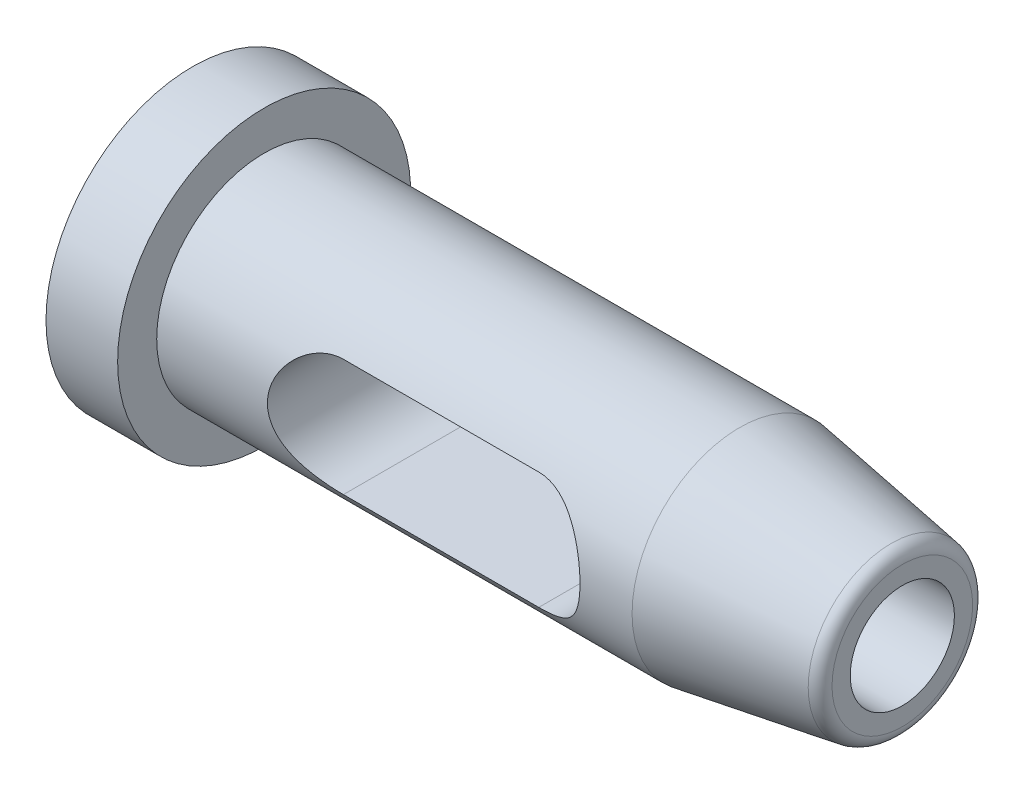
SolidWorks part; units mm, degrees
material "Plain Carbon Steel"
ref_plane "Front Plane" through (0, 0, 0) normal (0, 0, 1) x (1, 0, 0)
ref_plane "Top Plane" through (0, 0, 0) normal (0, 1, 0) x (1, 0, 0)
ref_plane "Right Plane" through (0, 0, 0) normal (1, 0, 0) x (0, 0, -1)
sketch "Holder Profile Sketch" plane through (0, 0, 0) normal (0, 0, 1) x (1, 0, 0)
  line L0 (-42.8298, 0) -> (109, 0) construction
  line L5 (0, 0) -> (0, 22.5)
  line L6 (0, 22.5) -> (11, 22.5)
  line L7 (11, 22.5) -> (11, 16.5)
  line L8 (11, 16.5) -> (84, 16.5)
  line L9 (84, 16.5) -> (109, 12.5)
  line L10 (109, 12.5) -> (109, 0)
  line L11 (109, 0) -> (0, 0)
  dimension "D1" = 11
  dimension "D2" = 25
  dimension "D3" = 98
  dimension "D4" = 22.5
  dimension "D5" = 12.5
  dimension "D6" = 16.5
revolve "Holder Body Revolve" add sketch "Holder Profile Sketch" angle 360 about L0
sketch "Side Window Sketch" plane through (0, 0, 0) normal (0, 0, 1) x (1, 0, 0)
  line L0 (37, 0) -> (67, 0) construction
  line L1 (37, 9) -> (67, 9)
  line L2 (37, -9) -> (67, -9)
  arc A0 (37, 9) -> (37, -9) centre (37, 0) ccw
  arc A1 (67, -9) -> (67, 9) centre (67, 0) ccw
  point P3 (52, 0)
  dimension "D3" = 9
  dimension "D1" = 26
  dimension "D2" = 30
extrude "Side Window Cut" cut sketch "Side Window Sketch" against normal through all both and the other way through all
fillet "Edge Fillet R2" radius 2 1 edges at (109, 0, 12.5)
sketch "Bore Sketch Ø16" plane through (109, 0, 0) normal (1, 0, 0) x (0, 0, -1)
  circle A0 centre (0, 0) radius 8
  dimension "D1" = 16
extrude "Bore Ø16" cut sketch "Bore Sketch Ø16" against normal up to next
